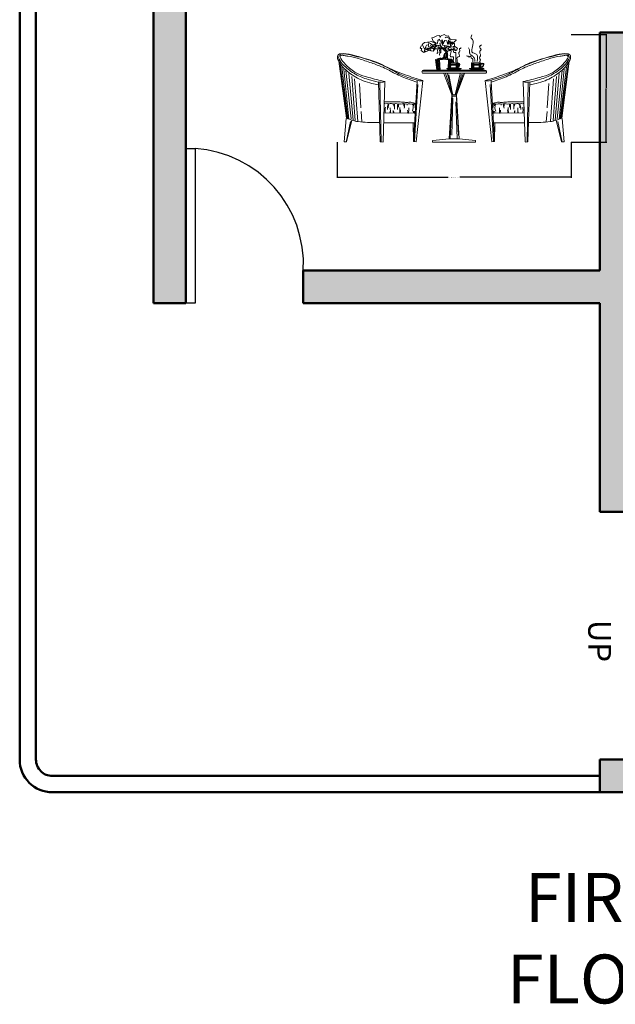
# Model space of a CAD drawing. Units: inches. Extents: x 1771 to 3025, y 319 to 889.
# Tile 13 of 35: x 2219 to 2402, y 319 to 621. Entities that reach past the tile are written whole.
import ezdxf

# ---------------------------------------------------------------- set-up
doc = ezdxf.new("R2010")
doc.units = ezdxf.units.IN
doc.header["$MEASUREMENT"] = 0
for name, color, linetype, lineweight in [('A-ANNO-DIMS', 2, 'Continuous', 18), ('A-AREA-IDEN', 241, 'Continuous', 25), ('A-DOOR', 4, 'Continuous', 25), ('A-FURN', 8, 'Continuous', 18), ('A-WALL', 7, 'Continuous', 50), ('A-WALL-PATT', 254, 'Continuous', 13)]:
    doc.layers.add(name, color=color, linetype=linetype, lineweight=lineweight)
doc.styles.get("Standard").update_dxf_attribs({"font": 'arial.ttf'})
doc.dimstyles.get("Standard").update_dxf_attribs({"dimtxt": 0.18, "dimasz": 0.18, "dimexe": 0.18, "dimexo": 0.0625, "dimgap": 0.09, "dimtad": 0, "dimtih": 1, "dimtoh": 1, "dimdec": 4, "dimzin": 0, "dimdsep": 46, "dimtxsty": 'Standard', "dimcen": 0.09, "dimadec": 0, "dimazin": 0, "dimtfac": 1, "dimtdec": 4, "dimtofl": 0, "dimtmove": 0, "dimatfit": 3, "dimfxl": 1, "dimtolj": 1, "dimtzin": 0, "dimarcsym": 0})

# ---------------------------------------------------------------- blocks, each defined once
blk = doc.blocks.new('A$C7D4176DC')
for p, q in [((850.3, 971.5), (825.9, 951.9)), ((879.3, 973.4), (850.3, 971.5)), ((889.6, 974.3), (879.3, 973.4)), ((886.8, 949.1), (892.4, 968.7)), ((914, 980.9), (889.6, 974.3)), ((892.4, 968.7), (908.4, 962.2)), ((908.4, 962.2), (934.6, 940.6)), ((947.7, 967.8), (914, 980.9)), ((936.5, 1019.3), (919.6, 1018.3)), ((919.6, 1018.3), (933.7, 984.6)), ((933.7, 984.6), (961.8, 966.8)), ((969.3, 1036.1), (936.5, 1019.3)), ((958, 965.9), (946.8, 953.7)), ((961.8, 966.8), (976.7, 961.2)), ((994.5, 1040.8), (969.3, 1036.1)), ((976.7, 961.2), (980.5, 991.2)), ((980.5, 991.2), (994.5, 1005.2)), ((1000.2, 1022.1), (994.5, 1040.8)), ((994.5, 1005.2), (999.2, 992.1)), ((999.2, 992.1), (1006.7, 983.7)), ((999.2, 965.9), (1016.1, 967.8)), ((1003, 952.8), (999.2, 965.9)), ((1008.6, 1036.1), (1000.2, 1022.1)), ((1006.7, 983.7), (1022.6, 987.4)), ((1010.5, 1037.1), (1041.4, 1048.3)), ((1022.6, 987.4), (1015.2, 989.3)), ((1016.1, 967.8), (1017, 970.6)), ((1029.2, 982.8), (1017, 998.7)), ((1017, 998.7), (1017, 981.8)), ((1017, 981.8), (1024.5, 946.2)), ((1017, 970.6), (1037.6, 969.7)), ((1032, 956.5), (1029.2, 982.8)), ((1042.3, 979.9), (1032, 956.5)), ((1037.6, 969.7), (1033, 971.5)), ((1041.4, 1048.3), (1064.8, 1036.1)), ((1047.9, 992.1), (1042.3, 979.9)), ((1066.7, 989.3), (1047.9, 992.1)), ((1051.7, 1018.3), (1059.2, 1023)), ((1059.2, 1023), (1090.1, 1013.6)), ((1064.8, 1036.1), (1077, 1034.2)), ((1075.1, 953.7), (1066.7, 989.3)), ((1077, 1034.2), (1084.5, 1035.2)), ((1081.7, 994), (1079.8, 959.4)), ((1095.7, 976.2), (1081.7, 994)), ((1084.5, 1035.2), (1097.6, 1007.1)), ((1103.2, 982.8), (1084.5, 969.7)), ((1084.5, 969.7), (1084.5, 959.4)), ((1091, 1009.9), (1088.2, 1005.2)), ((1088.2, 1005.2), (1104.1, 1009)), ((1090.1, 1013.6), (1091, 1009.9)), ((1104.1, 1009), (1091, 1005.2)), ((1091, 1005.2), (1100.4, 1003.4)), ((1121, 975.3), (1095.7, 976.2)), ((1100.4, 1003.4), (1103.2, 993.1)), ((1100.4, 971.5), (1103.2, 982.8)), ((1101.3, 940.6), (1100.4, 971.5)), ((1106, 966.8), (1104.1, 968.7)), ((1121, 969.7), (1106, 966.8)), ((1108.2, 1001.8), (1157.5, 996.8)), ((1119.1, 963.1), (1121, 969.7)), ((1127.6, 960.3), (1119.1, 963.1)), ((1132.2, 960.3), (1121, 975.3)), ((1137.9, 978.1), (1132.2, 960.3)), ((1151, 989.3), (1137.9, 978.1)), ((1159.4, 994), (1151, 989.3)), ((1157.5, 996.8), (1159.4, 994)), ((820.3, 941.6), (808.1, 920)), ((808.1, 920), (811.9, 913.5)), ((811.9, 913.5), (821.2, 911.6)), ((821.2, 911.6), (817.5, 893.8)), ((817.5, 893.8), (843.7, 875.1)), ((825.9, 951.9), (853.1, 902.3)), ((843.7, 875.1), (847.5, 880.7)), ((847.5, 897.6), (877.4, 906)), ((847.5, 880.7), (847.5, 897.6)), ((853.1, 902.3), (863.4, 931.3)), ((862.1, 880.4), (853.9, 886.5)), ((860.6, 917.2), (858.7, 916.3)), ((863.4, 917.2), (860.6, 917.2)), ((878.4, 916.3), (861.5, 919.1)), ((886.7, 892.7), (862.1, 880.4)), ((863.4, 931.3), (869, 944.4)), ((876.5, 911.6), (863.4, 917.2)), ((870.3, 898.8), (868.3, 907)), ((869, 944.4), (886.8, 949.1)), ((895, 892.7), (870.3, 898.8)), ((879.3, 906.9), (876.5, 911.6)), ((877.4, 906), (884.9, 905.1)), ((883.1, 912.5), (878.4, 916.3)), ((894.3, 912.5), (879.3, 906.9)), ((910.2, 917.2), (883.1, 912.5)), ((890.6, 924.7), (884, 950)), ((884.9, 905.1), (889.6, 903.2)), ((889.6, 903.2), (895.2, 901.3)), ((900.9, 928.5), (890.6, 924.7)), ((902.7, 916.3), (894.3, 912.5)), ((931.9, 888.6), (895, 892.7)), ((895.2, 901.3), (899, 917.2)), ((922.4, 927.5), (900.9, 928.5)), ((903.7, 927.5), (902.7, 916.3)), ((905.6, 928.5), (903.7, 927.5)), ((904.6, 923.8), (905.6, 928.5)), ((904.6, 920), (904.6, 923.8)), ((919.6, 920), (904.6, 920)), ((909.3, 913.2), (907.3, 892.7)), ((909.3, 940.6), (908.4, 947.2)), ((917.7, 936), (909.3, 940.6)), ((917.5, 890.6), (909.3, 890.6)), ((939.3, 910.7), (910.2, 917.2)), ((931.9, 888.6), (917.5, 890.6)), ((928, 933.1), (917.7, 936)), ((939.3, 913.5), (919.6, 920)), ((932.7, 929.4), (922.4, 927.5)), ((927.4, 947.9), (955.2, 956.5)), ((942.1, 925.7), (928, 933.1)), ((940.1, 909.1), (931.9, 888.6)), ((950.4, 907), (931.9, 888.6)), ((941.1, 929.4), (932.7, 929.4)), ((934.6, 940.6), (938.3, 938.8)), ((985.2, 912.5), (939.3, 910.7)), ((951.5, 911.6), (941.1, 929.4)), ((950.5, 917.2), (942.1, 925.7)), ((946.8, 953.7), (945.8, 946.2)), ((945.8, 946.2), (971.1, 945.3)), ((955.2, 940.6), (946.8, 924.7)), ((946.8, 924.7), (951.5, 918.2)), ((1026.4, 913.5), (950.4, 907.4)), ((952.4, 910.7), (950.5, 917.2)), ((959.9, 938.8), (951.5, 925.7)), ((951.5, 925.7), (954.3, 912.5)), ((951.5, 918.2), (951.5, 911.6)), ((954.3, 909.7), (955.2, 940.6)), ((954.3, 912.5), (954.3, 909.7)), ((955.2, 956.5), (961.8, 934.1)), ((986.1, 943.4), (960.8, 940.6)), ((961.8, 934.1), (984.2, 923.8)), ((967.4, 939.2), (999.2, 945.3)), ((977.6, 875.3), (973.4, 867.6)), ((973.4, 867.6), (973.4, 860.6)), ((976.2, 896.9), (974.8, 892)), ((974.8, 892), (977.6, 877.4)), ((978.3, 903.2), (976.2, 896.9)), ((977.6, 912.2), (978.3, 903.2)), ((977.6, 877.4), (977.6, 875.3)), ((984.2, 923.8), (995.5, 925.7)), ((988.9, 914.4), (985.2, 912.5)), ((989.9, 930.3), (986.1, 943.4)), ((991.7, 916.3), (988.9, 914.4)), ((989.5, 915.7), (998.5, 919.9)), ((995.5, 925.7), (989.9, 930.3)), ((1005.8, 917.2), (991.7, 916.3)), ((998.5, 904.6), (995.7, 898.3)), ((995.7, 898.3), (999.9, 878.8)), ((997.1, 872.5), (996.4, 855.8)), ((999.9, 878.8), (997.1, 872.5)), ((998.5, 919.9), (1000.6, 912.2)), ((1000.6, 912.2), (998.5, 904.6)), ((999.2, 945.3), (1003, 952.8)), ((1002, 948.1), (1001.1, 940.6)), ((1001.1, 940.6), (1006.7, 926.6)), ((1012.3, 931.3), (1002, 948.1)), ((1006.9, 906), (1004.1, 898.3)), ((1004.1, 898.3), (1009, 894.8)), ((1008.3, 872.5), (1004.8, 871.8)), ((1007.7, 920), (1005.8, 917.2)), ((1006.7, 926.6), (1011.4, 921.9)), ((1011.8, 911.5), (1006.9, 906)), ((1006.9, 911.5), (1030.6, 908)), ((1009, 889.2), (1006.9, 877.4)), ((1006.9, 877.4), (1008.3, 872.5)), ((1027.3, 916.3), (1007.7, 920)), ((1009, 894.8), (1009, 889.2)), ((1009.7, 920.6), (1011.8, 911.5)), ((1011.4, 921.9), (1025.5, 914.4)), ((1021.7, 921.9), (1012.3, 931.3)), ((1033, 919.1), (1021.7, 921.9)), ((1024.5, 946.2), (1082.6, 936)), ((1025.5, 914.4), (1048.9, 908.8)), ((1030.6, 908), (1036.9, 901.1)), ((1046.7, 908.7), (1033, 919.1)), ((1036.9, 901.1), (1049.5, 899)), ((1039, 899), (1045.3, 891.3)), ((1049.5, 899), (1039, 899)), ((1047.9, 941.6), (1043.3, 939.7)), ((1043.3, 939.7), (1048.9, 920)), ((1050.9, 864.8), (1044.6, 864.1)), ((1045.3, 891.3), (1052.3, 886.4)), ((1055.4, 914.4), (1047.9, 941.6)), ((1048.9, 920), (1049.8, 910.7)), ((1048.9, 908.8), (1076, 881.7)), ((1049.8, 910.7), (1050.8, 902.3)), ((1050.8, 902.3), (1060.1, 872.3)), ((1058.2, 880.7), (1050.8, 894.8)), ((1055.8, 873.9), (1050.9, 864.8)), ((1052.3, 886.4), (1057.9, 876.7)), ((1067.6, 934.1), (1054.5, 910.7)), ((1054.5, 910.7), (1054.5, 898.5)), ((1054.5, 898.5), (1059.9, 896.9)), ((1056.4, 890.1), (1055.4, 914.4)), ((1056.4, 905.1), (1055.4, 895.7)), ((1055.4, 895.7), (1057.3, 892)), ((1057.9, 876.7), (1055.8, 873.9)), ((1061.1, 918.2), (1056.4, 905.1)), ((1064.4, 865.4), (1056.9, 822.4)), ((1060.1, 872.3), (1058.2, 880.7)), ((1069.5, 859.2), (1059.2, 870.4)), ((1064.8, 923.8), (1061.1, 918.2)), ((1065.7, 884.5), (1061.1, 875.1)), ((1061.1, 875.1), (1061.1, 857.3)), ((1067.6, 929.4), (1064.8, 927.5)), ((1066.7, 926.6), (1064.8, 923.8)), ((1074.2, 859.2), (1065.7, 884.5)), ((1070.4, 864.8), (1065.7, 823.6)), ((1089.2, 931.3), (1066.7, 926.6)), ((1084.5, 932.2), (1067.6, 929.4)), ((1070.4, 862.9), (1067.6, 890.1)), ((1076, 851.7), (1070.4, 864.8)), ((1076, 881.7), (1071.4, 876)), ((1071.4, 876), (1073.2, 863.9)), ((1072.3, 910), (1078.2, 913)), ((1091.3, 904.2), (1072.3, 910)), ((1076.7, 886.6), (1073.8, 883.7)), ((1079.8, 959.4), (1075.1, 953.7)), ((1097.2, 895.4), (1076.7, 886.6)), ((1078.2, 913), (1100.1, 932)), ((1082.6, 936), (1096.7, 928.5)), ((1084.5, 959.4), (1127.6, 960.3)), ((1098.6, 893.9), (1089.9, 904.2)), ((1113.3, 911.5), (1091.3, 904.2)), ((1096.7, 928.5), (1101.3, 922.8)), ((1100.1, 932), (1097.2, 927.6)), ((1097.2, 927.6), (1117.7, 930.5)), ((1113.3, 902.7), (1097.2, 895.4)), ((1113.3, 899.8), (1098.6, 893.9)), ((1101.3, 922.8), (1111.6, 941.6)), ((1111.6, 941.6), (1101.3, 940.6)), ((1122.1, 904.2), (1113.3, 911.5)), ((1127.9, 901.3), (1113.3, 899.8)), ((1117.7, 930.5), (1139.6, 927.6)), ((1138.2, 914.4), (1122.1, 904.2)), ((1138.2, 895.4), (1127.9, 901.3)), ((1129.4, 933.4), (1145.5, 933.4)), ((1144, 908.6), (1138.2, 914.4)), ((1151.3, 895.4), (1138.2, 895.4)), ((1151.3, 891), (1144, 908.6)), ((1145.5, 933.4), (1160.1, 923.2)), ((1166, 901.3), (1151.3, 891)), ((1160.1, 923.2), (1166, 918.8)), ((1166, 918.8), (1170.4, 917.3)), ((1170.4, 917.3), (1166, 901.3)), ((13.4, 788.5), (86.9, 232)), ((968.4, 700.9), (955.2, 806.2)), ((955.2, 806.2), (1126.5, 803.3)), ((959.3, 806.1), (972.5, 701.9)), ((965.6, 806.1), (976.7, 700.5)), ((976.6, 787.5), (968.6, 786.7)), ((968.6, 786.7), (971.7, 756.8)), ((991.6, 820.2), (969.9, 808.3)), ((975.3, 805.4), (983, 701.2)), ((979.7, 757.6), (976.6, 787.5)), ((979.4, 811.3), (977.9, 801.1)), ((991.8, 816.4), (978.6, 806.2)), ((985.8, 805.4), (990.6, 701.9)), ((1016.7, 816), (991.6, 820.2)), ((1003.5, 807.6), (991.8, 816.4)), ((996.2, 804.1), (1001.1, 701.9)), ((996.4, 855.8), (996.4, 850.9)), ((996.4, 850.9), (997.8, 845.3)), ((1009.4, 822.3), (1002, 816.4)), ((1002, 816.4), (1054.7, 813.5)), ((1013.7, 810.6), (1003.5, 807.6)), ((1041.6, 819.3), (1013.7, 810.6)), ((1060.6, 835.8), (1015.2, 815.4)), ((1022.3, 819.5), (1016.7, 816)), ((1024.4, 819.5), (1022.3, 819.5)), ((1026.5, 819.5), (1024.4, 819.5)), ((1029.9, 828.6), (1026.5, 819.5)), ((1032, 829.3), (1029.9, 828.6)), ((1033.4, 828.6), (1032, 829.3)), ((1036.9, 832), (1033.4, 828.6)), ((1037.6, 834.1), (1036.9, 832)), ((1044.5, 828.1), (1037.2, 822.3)), ((1037.2, 822.3), (1041.6, 819.3)), ((1039, 850.9), (1037.6, 836.2)), ((1037.6, 836.2), (1037.6, 834.1)), ((1039.7, 853), (1039, 850.9)), ((1044.6, 864.1), (1039.7, 853)), ((1048.9, 832.5), (1044.5, 828.1)), ((1048.1, 856.4), (1045.3, 850.2)), ((1045.3, 850.2), (1045.3, 839)), ((1045.3, 839), (1048.1, 841.1)), ((1048.1, 841.1), (1048.8, 853.7)), ((1048.8, 853.7), (1048.8, 857.1)), ((1057.7, 829.6), (1048.9, 832.5)), ((1049.8, 817.1), (1076, 851.7)), ((1051.7, 827.4), (1049.8, 817.1)), ((1054.7, 813.5), (1057.7, 829.6)), ((1061.1, 857.3), (1064.8, 853.6)), ((1064.8, 853.6), (1069.5, 859.2)), ((1065.7, 823.6), (1077, 814.3)), ((1066.4, 817.9), (1066.4, 812)), ((1066.4, 812), (1075.2, 806.2)), ((1074.2, 829.2), (1070.4, 862.9)), ((1073.2, 863.9), (1074.2, 859.2)), ((1075.2, 806.2), (1073.8, 812)), ((1073.8, 812), (1114.7, 807.6)), ((1077, 814.3), (1074.2, 829.2)), ((1098.2, 804.7), (1077.7, 804.7)), ((1083.8, 803.4), (1080.4, 718.8)), ((1088.8, 774.3), (1088.8, 724.7)), ((1179, 774.3), (1088.8, 774.3)), ((1090.9, 774.1), (1090.9, 725.1)), ((1093.6, 804.7), (1091.9, 774.3)), ((1093.9, 773.8), (1093.9, 725.1)), ((1114.7, 807.6), (1097.2, 801.8)), ((1098.4, 774.1), (1098.4, 724.9)), ((1104, 802), (1101.5, 774.3)), ((1104.1, 773.8), (1104.1, 763.6)), ((1110.9, 799.9), (1108, 774.3)), ((1117.9, 803.4), (1113.7, 774.3)), ((1125, 803.3), (1120, 774.3)), ((1158.2, 773.8), (1158.2, 725.1)), ((1164.1, 773.8), (1164.1, 724.9)), ((1168.6, 774.3), (1168.6, 725.4)), ((1172.9, 774.1), (1172.9, 767.4)), ((1175.9, 774.1), (1175.9, 767.3)), ((1178, 773.8), (1178, 767.2)), ((1179, 767.3), (1179, 774.3)), ((1309.2, 774.3), (1309.2, 724.7)), ((1399.4, 774.3), (1309.2, 774.3)), ((1311, 774.3), (1311, 725)), ((1313.8, 774.6), (1313.8, 724)), ((1318.3, 774.3), (1318.3, 725.2)), ((1324.3, 774.1), (1324.3, 725.5)), ((1331.2, 774.1), (1331.2, 725)), ((1383.9, 774.1), (1383.9, 725.2)), ((1389.2, 774.1), (1389.2, 724.8)), ((1393.7, 774.1), (1393.7, 724.5)), ((1396.6, 774.1), (1396.6, 724.8)), ((1398.3, 774.1), (1398.3, 724.8)), ((1399.4, 724.7), (1399.4, 774.3)), ((2261.7, 788.5), (2188.2, 232)), ((24.7, 755.7), (94.7, 231.2)), ((41.1, 733.1), (100.8, 229.1)), ((61.7, 710.4), (111.1, 223)), ((82.3, 698.1), (131.7, 227.1)), ((1452.4, 690.9), (826.8, 690.9)), ((1438.5, 700.9), (838.5, 700.9)), ((1107.4, 700.9), (968.4, 700.9)), ((971.7, 756.8), (979.7, 757.6)), ((1206.9, 718.8), (1068.5, 718.8)), ((1205.1, 715), (1070.7, 715)), ((1079.9, 707.4), (1079.6, 701.2)), ((1192.2, 706.1), (1080.1, 706.6)), ((1191.5, 704.8), (1081.7, 704.8)), ((1083.3, 700.5), (1083.3, 704.5)), ((1100.8, 759), (1088.8, 759)), ((1088.8, 724.7), (1179, 724.7)), ((1100.8, 751.4), (1090.1, 751.4)), ((1093.2, 718.3), (1093.2, 724.5)), ((1100.8, 763.6), (1100.8, 747.6)), ((1107.3, 763.6), (1100.8, 763.6)), ((1100.8, 747.6), (1107.3, 747.6)), ((1101.3, 745), (1101.3, 740.5)), ((1107.3, 745), (1101.3, 745)), ((1101.3, 740.5), (1107.3, 740.5)), ((1104.1, 747.6), (1104.1, 745)), ((1104.1, 740.5), (1104.1, 724.7)), ((1107.3, 747.6), (1107.3, 763.6)), ((1179, 759), (1107.3, 759)), ((1179, 751.4), (1107.3, 751.4)), ((1107.3, 740.5), (1107.3, 745)), ((1172.9, 762.7), (1172.9, 734.9)), ((1172.9, 732.2), (1172.9, 725.1)), ((1173.3, 725.1), (1173.3, 718.3)), ((1175.9, 762.6), (1175.9, 734.6)), ((1175.9, 731.8), (1175.9, 724.6)), ((1178.3, 762.6), (1178.3, 734.8)), ((1178.3, 731.3), (1178.3, 725.1)), ((1179, 734.4), (1179, 762.7)), ((1179, 724.7), (1179, 731.4)), ((1189, 704.5), (1189, 700.5)), ((1427.3, 718.8), (1288.9, 718.8)), ((1425.4, 715), (1291, 715)), ((1412.6, 706.1), (1300.5, 706.6)), ((1411.9, 704.8), (1302.1, 704.8)), ((1303.7, 700.5), (1303.7, 704.5)), ((1319.1, 759), (1309.2, 759)), ((1309.2, 724.7), (1399.4, 724.7)), ((1319.1, 751.4), (1310.5, 751.4)), ((1313.5, 718.3), (1313.5, 724.5)), ((1319.1, 764.9), (1319.1, 742.2)), ((1323.5, 764.9), (1319.1, 764.9)), ((1319.1, 742.2), (1323.5, 742.2)), ((1319.8, 739.2), (1319.8, 735.6)), ((1322.7, 739.2), (1319.8, 739.2)), ((1319.8, 735.6), (1322.7, 735.6)), ((1322.7, 735.6), (1322.7, 739.2)), ((1323.5, 742.2), (1323.5, 764.9)), ((1399.4, 759), (1323.5, 759)), ((1399.4, 751.4), (1323.5, 751.4)), ((1393.7, 725.1), (1393.7, 718.3)), ((1409.4, 704.5), (1409.4, 700.5)), ((2192.8, 698.1), (2143.4, 227.1)), ((2213.3, 710.4), (2163.9, 223)), ((2233.9, 733.1), (2174.2, 229.1)), ((2250.4, 755.7), (2180.4, 231.2)), ((111.1, 669.3), (152.3, 214.7)), ((137.9, 640.5), (170.8, 210.6)), ((166.7, 615.8), (197.6, 202.4)), ((398.7, 587.3), (417.4, 0.9)), ((413.7, 579.8), (424.7, 0.9)), ((462.3, 591), (443.8, 0.9)), ((776.4, 594.8), (742.7, 4.4)), ((795.6, 597.2), (767.4, 606)), ((832.5, 602.2), (768.9, 2.8)), ((772.6, 598.5), (776.4, 598.5)), ((825, 598.5), (795.6, 597.2)), ((1438.5, 670.9), (838.5, 670.9)), ((1037.2, 670.1), (1115.4, 459.8)), ((1054.9, 670.7), (1122.1, 460.1)), ((1073, 665.2), (1125.7, 463.7)), ((1085.8, 656.2), (1122.1, 471)), ((1198.4, 667), (1147.5, 461.9)), ((1209.3, 659.8), (1156.6, 467.4)), ((1227.5, 665.2), (1160.2, 467.4)), ((1239.7, 670.1), (1161.5, 459.8)), ((1442.6, 602.2), (1506.2, 2.8)), ((1450.1, 598.5), (1479.4, 597.2)), ((1479.4, 597.2), (1507.7, 606)), ((1502.4, 598.5), (1498.7, 598.5)), ((1498.7, 594.8), (1532.3, 4.4)), ((1812.8, 591), (1831.2, 0.9)), ((1861.4, 579.8), (1850.3, 0.9)), ((1876.4, 587.3), (1857.7, 0.9)), ((2108.4, 615.8), (2077.5, 202.4)), ((2137.2, 640.5), (2104.3, 210.6)), ((2163.9, 669.3), (2122.8, 214.7)), ((214, 572.6), (228.4, 334)), ((783.9, 560.6), (752.8, 5.4)), ((1491.2, 560.6), (1522.3, 5.4)), ((2061, 572.6), (2046.6, 334)), ((1115.4, 459.8), (1088.3, 33.1)), ((1118.5, 442), (1100.3, 33.5)), ((1163.9, 447.4), (1114.8, 447.4)), ((1161.5, 459.8), (1115.4, 459.8)), ((1123.9, 427.4), (1116.6, 68)), ((1154.8, 393), (1167.5, 35.4)), ((1160.2, 436.5), (1180.2, 66.2)), ((1161.5, 459.8), (1188.6, 33.1)), ((230.5, 299.1), (238.7, 196.2)), ((465.7, 375.8), (456.5, 375.8)), ((484.1, 377.3), (471.9, 374.3)), ((499.5, 372.7), (484.1, 377.3)), ((508.7, 374.3), (499.5, 372.7)), ((513.3, 375.8), (508.7, 374.3)), ((525.5, 375.8), (513.3, 375.8)), ((531.7, 374.3), (525.5, 375.8)), ((543.9, 374.3), (531.7, 374.3)), ((547, 371.2), (543.9, 374.3)), ((567, 375.8), (547, 371.2)), ((582.3, 374.3), (567, 375.8)), ((593, 371.2), (590, 374.3)), ((606.8, 372.7), (593, 371.2)), ((611.4, 369.7), (606.8, 372.7)), ((629.8, 372.7), (611.4, 369.7)), ((636, 374.3), (629.8, 372.7)), ((643.6, 375.8), (636, 374.3)), ((648.2, 372.7), (643.6, 375.8)), ((659, 372.7), (648.2, 372.7)), ((677.4, 371.2), (659, 372.7)), ((678.9, 371.2), (678.9, 359)), ((697.3, 374.3), (685.1, 372.7)), ((706.5, 374.3), (697.3, 374.3)), ((715.7, 371.2), (706.5, 374.3)), ((729.5, 372.7), (715.7, 371.2)), ((740.3, 374.3), (729.5, 368.2)), ((729.5, 368.2), (729.5, 372.7)), ((747.9, 374.3), (740.3, 374.3)), ((751, 369.7), (747.9, 374.3)), ((760.2, 374.3), (751, 369.7)), ((1514.9, 374.3), (1524.1, 369.7)), ((1524.1, 369.7), (1527.1, 374.3)), ((1527.1, 374.3), (1534.8, 374.3)), ((1534.8, 374.3), (1545.5, 368.2)), ((1545.5, 372.7), (1559.3, 371.2)), ((1545.5, 368.2), (1545.5, 372.7)), ((1559.3, 371.2), (1568.5, 374.3)), ((1568.5, 374.3), (1577.7, 374.3)), ((1577.7, 374.3), (1590, 372.7)), ((1596.2, 371.2), (1596.2, 359)), ((1597.7, 371.2), (1616.1, 372.7)), ((1616.1, 372.7), (1626.8, 372.7)), ((1626.8, 372.7), (1631.4, 375.8)), ((1631.4, 375.8), (1639.1, 374.3)), ((1639.1, 374.3), (1645.2, 372.7)), ((1645.2, 372.7), (1663.6, 369.7)), ((1663.6, 369.7), (1668.2, 372.7)), ((1668.2, 372.7), (1682, 371.2)), ((1682, 371.2), (1685.1, 374.3)), ((1692.8, 374.3), (1708.1, 375.8)), ((1708.1, 375.8), (1728.1, 371.2)), ((1728.1, 371.2), (1731.1, 374.3)), ((1731.1, 374.3), (1743.4, 374.3)), ((1743.4, 374.3), (1749.5, 375.8)), ((1749.5, 375.8), (1761.8, 375.8)), ((1761.8, 375.8), (1766.4, 374.3)), ((1766.4, 374.3), (1775.6, 372.7)), ((1775.6, 372.7), (1790.9, 377.3)), ((1790.9, 377.3), (1803.2, 374.3)), ((1809.3, 375.8), (1818.5, 375.8)), ((2044.6, 299.1), (2036.3, 196.2)), ((84, 230.1), (64.2, 2.8)), ((126, 200.5), (84, 0.3)), ((140.9, 212.8), (88.9, 2.8)), ((756.8, 280.8), (451.1, 284.6)), ((1518.3, 280.8), (1824, 284.6)), ((2134.2, 212.8), (2186.2, 2.8)), ((2149.1, 200.5), (2191.1, 0.3)), ((2191.1, 230.1), (2210.9, 2.8)), ((447.3, 187.5), (757.7, 187.5)), ((739, 187.5), (742.7, 4.4)), ((1827.8, 187.5), (1517.4, 187.5)), ((1536.1, 187.5), (1532.3, 4.4)), ((64.2, 2.8), (88.9, 2.8)), ((417.4, 0.9), (443.8, 0)), ((742.7, 4.4), (746.5, 38)), ((742.7, 4.4), (768.9, 2.8)), ((927.1, 15), (927.1, 0)), ((1088.3, 33.1), (929, 15)), ((1187.5, 31.7), (1087.6, 31.7)), ((1188.6, 33.1), (1348, 15)), ((1348, 15), (1348, 0)), ((1532.3, 4.4), (1506.2, 2.8)), ((1532.3, 4.4), (1528.6, 38)), ((1857.7, 0.9), (1831.3, 0)), ((2210.9, 2.8), (2186.2, 2.8)), ((1348, 0), (927.1, 0))]:
    blk.add_line(p, q)
for centre, radius, start, end in [((838.2, 685.9), 15, 89.02539, 270.97461), ((1069.4, 716.9), 2.21, 114.75071, 294.8305), ((1059.6, 691.4), 25.9, 31.12717, 65.45392), ((1208.6, 696.5), 19, 99.79621, 154.31096), ((1206.2, 716.7), 1.95, 244.55032, 96.50843), ((1289.8, 716.9), 2.21, 114.75071, 294.8305), ((1280, 691.4), 25.9, 31.12717, 65.45392), ((1429, 696.5), 19, 99.79621, 154.31096), ((1426.6, 716.7), 1.95, 244.55032, 96.50843), ((1440.2, 685.9), 15.1, 263.50595, 96.49405), ((421.9, 675.7), 92.7, 253.90068, 295.36386), ((1853.1, 675.7), 92.7, 244.63614, 286.09932), ((665.2, 310.8), 200.4, 171.53233, 187.34342), ((631.7, 325.3), 145, 160.46362, 183.26427), ((661.3, 321.8), 167.8, 162.1481, 175.52768), ((522.1, 292), 10.6, 155.04372, 216.38582), ((746.2, 323.3), 231.2, 177.65923, 189.89094), ((596.6, 305.3), 53.4, 177.23164, 203.39317), ((-475.8, 101.1), 1042.4, 10.14258, 11.10952), ((592, 359.5), 42.9, 161.29008, 193.50095), ((755.4, 341.1), 200.6, 170.95256, 185.34949), ((841.5, 337.8), 255.8, 172.03905, 184.65389), ((943.9, 345.9), 348.8, 175.42446, 180.75439), ((484.6, 319.5), 124.8, 342.71731, 8.30681), ((204.5, 341.5), 411.6, 351.83053, 356.14259), ((590.6, 356.2), 56.7, 354.25823, 16.89433), ((579.3, 354.7), 74.8, 340.32989, 13.94105), ((645.6, 301.5), 39.5, 333.88539, 14.90767), ((494.8, 326.9), 201, 346.57929, 1.64099), ((619.9, 341.7), 118.4, 339.52102, 14.35705), ((682.4, 301.4), 59.8, 341.0378, 359.49279), ((693.6, 357.6), 48.4, 353.58471, 16.22063), ((616.9, 303.9), 135.6, 349.74606, 359.61704), ((689.2, 351.2), 68.2, 347.09902, 16.48344), ((1585.8, 351.2), 68.2, 163.51656, 192.90098), ((1658.2, 303.9), 135.6, 180.38296, 190.25394), ((1592.7, 301.4), 59.8, 180.50721, 198.9622), ((1581.5, 357.6), 48.4, 163.77937, 186.41529), ((1655.1, 341.7), 118.4, 165.64295, 200.47898), ((1780.3, 326.9), 201, 178.35901, 193.42071), ((1629.4, 301.5), 39.5, 165.09233, 206.11461), ((1695.8, 354.7), 74.8, 166.05895, 199.67011), ((1684.4, 356.2), 56.7, 163.10567, 185.74177), ((2070.6, 341.5), 411.6, 183.85741, 188.16947), ((1790.4, 319.5), 124.8, 171.69319, 197.28269), ((1331.2, 345.9), 348.8, 359.24561, 4.57554), ((1433.6, 337.8), 255.8, 355.34611, 7.96095), ((1519.7, 341.1), 200.6, 354.65051, 9.04744), ((1683.1, 359.5), 42.9, 346.49905, 18.70992), ((2750.9, 101.1), 1042.4, 168.89048, 169.85742), ((1678.5, 305.3), 53.4, 336.60683, 2.76836), ((1528.9, 323.3), 231.2, 350.10906, 2.34077), ((1753, 292), 10.6, 323.61418, 24.95628), ((1613.7, 321.8), 167.8, 4.47232, 17.8519), ((1643.3, 325.3), 145, 356.73573, 19.53638), ((1609.9, 310.8), 200.4, 352.65658, 8.46767)]:
    blk.add_arc(centre, radius, start, end)
for points, knots in [([(1154.2, 782.2), (1154.8, 800.5), (1155.7, 825.5), (1152.5, 852.8), (1161, 880.4), (1126, 866.1), (1137.2, 896.5), (1131.8, 923.4), (1156.8, 968.1), (1113.4, 971.1), (1116.9, 957), (1118.7, 949.8)], [0, 0, 0, 0, 53.324624, 72.369114, 91.413604, 110.471764, 134.594802, 149.830446, 204.42477, 220.941926, 238.716972, 238.716972, 238.716972, 238.716972]), ([(1361.4, 785.9), (1364, 797.1), (1369.1, 819), (1366.1, 867.4), (1305.9, 865.7), (1312.3, 906.5), (1315.7, 942.7), (1336.1, 991.6), (1296, 1015.4), (1304.6, 1034), (1310, 1045.7)], [0, 0, 0, 0, 35.255511, 69.327341, 124.802742, 145.944632, 176.486081, 244.459642, 263.687549, 295.971636, 295.971636, 295.971636, 295.971636]), ([(832.5, 602.2), (773.3, 619.4), (552.4, 683.6), (381.9, 796.6), (-38, 894.8), (125.3, 689.4), (274.3, 633.7), (409.7, 603.5), (466, 591)], [0, 0, 0, 0, 179.241333, 669.878405, 853.517726, 978.360591, 1217.111989, 1387.04363, 1387.04363, 1387.04363, 1387.04363]), ([(1131.4, 779.6), (1130.3, 791.6), (1128.8, 807.5), (1135.2, 839.3), (1091.9, 821.5), (1105.3, 863.2), (1115.5, 900.9), (1079.7, 883.7), (1089.8, 909.5), (1078.6, 906.7), (1072.9, 905.3)], [0, 0, 0, 0, 39.358681, 52.054923, 76.195091, 115.553772, 137.137409, 158.736993, 171.43349, 184.13893, 184.13893, 184.13893, 184.13893]), ([(1166.9, 779.6), (1167.6, 787.2), (1168.9, 801.7), (1159.5, 831.3), (1208.7, 829.6), (1171.7, 871.4), (1202, 885.9), (1182.6, 918), (1207, 909.8), (1204.8, 918.7), (1203.8, 923.1)], [0, 0, 0, 0, 24.123038, 45.706674, 71.213394, 110.655389, 125.899008, 152.561192, 162.725628, 172.882723, 172.882723, 172.882723, 172.882723]), ([(1341.7, 785.9), (1340.2, 798.9), (1337.5, 822.1), (1313, 843.2), (1292.5, 855.8), (1286.2, 880.3), (1292.2, 903.3), (1280.3, 916.5), (1276.7, 920.3)], [0, 0, 0, 0, 37.360481, 67.270583, 93.998428, 104.993238, 141.362472, 156.467713, 156.467713, 156.467713, 156.467713]), ([(1385.6, 784.4), (1390.4, 789.9), (1401.4, 802.3), (1375.2, 822.1), (1401.7, 842.3), (1389.4, 864.6), (1386.5, 887), (1411.5, 904.8), (1373.5, 930.7), (1394.6, 942.4), (1403.7, 947.5)], [0, 0, 0, 0, 18.925439, 42.566292, 64.867201, 90.936936, 109.058775, 128.752565, 161.181972, 185.77482, 185.77482, 185.77482, 185.77482]), ([(1442.6, 602.2), (1501.7, 619.4), (1722.7, 683.6), (1893.2, 796.6), (2313.1, 894.8), (2149.7, 689.4), (2000.7, 633.7), (1865.4, 603.5), (1809.1, 591)], [0, 0, 0, 0, 179.241333, 669.878405, 853.517726, 978.360591, 1217.111989, 1387.04363, 1387.04363, 1387.04363, 1387.04363]), ([(398, 584.9), (364.8, 593.1), (288.2, 612.1), (173, 656.7), (78.3, 727.2), (27.8, 785.3), (-11.1, 856.8), (24.4, 860.7), (34.5, 861.8)], [0, 0, 0, 0, 102.450812, 236.341037, 372.740804, 434.264952, 500.538568, 526.867635, 526.867635, 526.867635, 526.867635]), ([(397.9, 557.5), (377.2, 562.2), (327.1, 573.6), (252, 594.7), (177.4, 633.5), (110.3, 676.9), (52.9, 727.5), (17.7, 778.4), (-3, 818.5), (1.2, 838.8), (2.4, 844.5)], [0, 0, 0, 0, 63.757158, 154.207673, 233.111021, 314.773872, 393.990027, 459.45949, 503.309158, 520.507412, 520.507412, 520.507412, 520.507412]), ([(774.4, 584.9), (749.6, 592.8), (676.5, 616.3), (565.4, 663.8), (449, 732.3), (326.3, 773), (214.5, 813.5), (122.5, 837.9), (67.5, 840.8), (36.8, 851.9), (27.3, 839.8), (24.3, 836)], [0, 0, 0, 0, 78.234212, 230.212389, 361.399227, 482.184421, 615.817971, 721.353317, 759.79292, 789.08251, 802.845503, 802.845503, 802.845503, 802.845503]), ([(778, 604.3), (747.1, 612.4), (671.2, 632.3), (544.7, 691), (406.7, 777.8), (262.4, 816.3), (152.4, 843.8), (83.7, 860.5), (45.9, 861.5), (34.5, 861.8)], [0, 0, 0, 0, 95.639299, 234.867324, 416.660896, 581.537135, 678.863317, 758.06805, 792.133261, 792.133261, 792.133261, 792.133261]), ([(1319.1, 782.9), (1321.9, 795.4), (1325.6, 812.1), (1309.5, 816.4), (1302.3, 822.2), (1305.8, 830.8), (1295.5, 845.6), (1286, 822.9), (1281.2, 839.2), (1270.5, 838.4), (1264.1, 839.6), (1260.1, 840.3)], [0, 0, 0, 0, 30.24085, 40.376736, 46.786017, 54.336911, 66.135106, 80.063877, 89.736225, 97.441532, 109.625491, 109.625491, 109.625491, 109.625491]), ([(1399.4, 767.3), (1402.9, 767.5), (1411.4, 768.1), (1432.6, 770.2), (1424.9, 746.9), (1419.3, 731), (1409, 728.9), (1399.9, 726.6), (1399.4, 728.7), (1399.4, 728.8)], [0, 0, 0, 0, 11.082717, 27.168464, 47.8303, 63.341794, 75.5235, 81.952599, 82.221535, 82.221535, 82.221535, 82.221535]), ([(1497.1, 604.3), (1528, 612.4), (1603.8, 632.3), (1730.4, 691), (1868.3, 777.8), (2012.7, 816.3), (2122.7, 843.8), (2191.4, 860.5), (2229.2, 861.5), (2240.6, 861.8)], [0, 0, 0, 0, 95.639299, 234.867324, 416.660896, 581.537135, 678.863317, 758.06805, 792.133261, 792.133261, 792.133261, 792.133261]), ([(1500.6, 584.9), (1525.5, 592.8), (1598.5, 616.3), (1709.7, 663.8), (1826.1, 732.3), (1948.7, 773), (2060.6, 813.5), (2152.5, 837.9), (2207.6, 840.8), (2238.3, 851.9), (2247.7, 839.8), (2250.7, 836)], [0, 0, 0, 0, 78.234212, 230.212389, 361.399227, 482.184421, 615.817971, 721.353317, 759.79292, 789.08251, 802.845503, 802.845503, 802.845503, 802.845503]), ([(1877.1, 584.9), (1910.3, 593.1), (1986.9, 612.1), (2102.1, 656.7), (2196.8, 727.2), (2247.3, 785.3), (2286.2, 856.8), (2250.7, 860.7), (2240.6, 861.8)], [0, 0, 0, 0, 102.450812, 236.341037, 372.740804, 434.264952, 500.538568, 526.867635, 526.867635, 526.867635, 526.867635]), ([(1877.1, 557.5), (1897.9, 562.2), (1947.9, 573.6), (2023.1, 594.7), (2097.7, 633.5), (2164.7, 676.9), (2222.2, 727.5), (2257.3, 778.4), (2278.1, 818.5), (2273.8, 838.8), (2272.7, 844.5)], [0, 0, 0, 0, 63.757158, 154.207673, 233.111021, 314.773872, 393.990027, 459.45949, 503.309158, 520.507412, 520.507412, 520.507412, 520.507412]), ([(1169.5, 767.6), (1169.1, 766.9), (1168.6, 765.8), (1168.5, 764.1), (1168.9, 763.4), (1169.1, 763)], [0, 0, 0, 0, 2.454471, 3.694729, 4.863756, 4.863756, 4.863756, 4.863756]), ([(1169.1, 763), (1172.8, 762.7), (1177.7, 762.3), (1183.6, 763.4), (1189.9, 762.9), (1187.4, 754.3), (1187.2, 747.1), (1184.4, 741.1), (1183.6, 734.2), (1179.1, 734.3), (1176.3, 734.5), (1173.7, 734.9), (1171.6, 734.9), (1169.1, 736.3), (1168.8, 734.4), (1168.7, 733.5), (1168.7, 732.9), (1169, 732.2), (1169.6, 732.2), (1169.9, 732.3)], [0, 0, 0, 0, 11.017731, 14.368752, 18.607743, 26.502791, 33.640107, 41.65747, 47.330925, 50.070533, 53.653147, 56.161165, 57.765785, 60.50412, 61.601302, 62.440841, 63.254964, 63.604793, 64.589255, 64.589255, 64.589255, 64.589255]), ([(1169.5, 767.6), (1173.2, 767.4), (1179.9, 766.9), (1197.8, 769.9), (1190.9, 747.3), (1187.7, 728.5), (1175.3, 732.4), (1169.7, 732.3), (1169.1, 732.2)], [0, 0, 0, 0, 11.640419, 20.980802, 45.0396, 57.043585, 71.929427, 73.92866, 73.92866, 73.92866, 73.92866]), ([(1180.5, 766.4), (1182.7, 766.7), (1186, 767.2), (1193.4, 764.4), (1189.7, 753.8), (1188.7, 747.3), (1188.2, 744.3)], [0, 0, 0, 0, 6.446326, 10.075492, 21.292554, 31.027811, 31.027811, 31.027811, 31.027811]), ([(1399.4, 760.8), (1402.3, 761.2), (1409.4, 762.1), (1423.2, 766.3), (1423.3, 753.9), (1420.3, 746.4), (1417.8, 735.7), (1409.3, 733.5), (1403.3, 729.7), (1400.4, 731.6), (1399.4, 732.3)], [0, 0, 0, 0, 9.652474, 22.996839, 29.518582, 40.146055, 49.702279, 58.739504, 65.130432, 68.539734, 68.539734, 68.539734, 68.539734]), ([(763.3, 374.3), (771.1, 374), (721.2, 391.5), (701, 387.4), (647.2, 387.1), (600.7, 394.2), (547.4, 391.8), (499.5, 394.7), (467.3, 394.3), (453.5, 394.2)], [0, 0, 0, 0, 23.359127, 69.600901, 112.546095, 167.952511, 215.499051, 270.735631, 312.147322, 312.147322, 312.147322, 312.147322]), ([(1511.8, 374.3), (1504, 374), (1553.9, 391.5), (1574.1, 387.4), (1627.8, 387.1), (1674.4, 394.2), (1727.7, 391.8), (1775.6, 394.7), (1807.8, 394.3), (1821.6, 394.2)], [0, 0, 0, 0, 23.359127, 69.600901, 112.546095, 167.952511, 215.499051, 270.735631, 312.147322, 312.147322, 312.147322, 312.147322]), ([(86.9, 232), (124.5, 219.1), (220.3, 186.2), (332, 194.5), (402.2, 190.3), (411.4, 189.7)], [0, 0, 0, 0, 118.259021, 301.591906, 329.266035, 329.266035, 329.266035, 329.266035]), ([(2188.2, 232), (2150.6, 219.1), (2054.8, 186.2), (1943.1, 194.5), (1872.9, 190.3), (1863.7, 189.7)], [0, 0, 0, 0, 118.259021, 301.591906, 329.266035, 329.266035, 329.266035, 329.266035])]:
    blk.add_open_spline(points, degree=3, knots=knots)
blk = doc.blocks.new('DOOR-36A')
blk.add_lwpolyline([(0, 47.37), (2.84, 47.37), (2.84, 0), (0, 0)], close=True)
blk.add_arc((0.47, 11.87), 35.58, 356.991, 86.1899)
blk = doc.blocks.new('*D44')
at = {"layer": 'A-ANNO-DIMS', "color": 0, "lineweight": -2, "transparency": 16777216}
for p, q in [((2316.52, 582.92), (2316.52, 572.04)), ((2388.29, 582.92), (2388.29, 572.04)), ((2316.7, 572.22), (2350.62, 572.22)), ((2388.11, 572.22), (2354.19, 572.22))]:
    blk.add_line(p, q, dxfattribs=at)
at = {"layer": 'A-ANNO-DIMS', "color": 0, "transparency": 16777216}
for points in [[(2316.7, 572.25), (2316.7, 572.19), (2316.52, 572.22)], [(2388.11, 572.25), (2388.11, 572.19), (2388.29, 572.22)]]:
    blk.add_solid(points, dxfattribs=at)
at = {"layer": 'Defpoints', "color": 0, "transparency": 16777216}
for p in [(2316.52, 582.99), (2388.29, 582.99), (2388.29, 572.22)]:
    blk.add_point(p, dxfattribs=at)
at = {"layer": 'A-ANNO-DIMS', "color": 0, "transparency": 16777216, "insert": (2352.4, 572.22), "char_height": 0.18, "attachment_point": 5}
blk.add_mtext('\\A1;COFFEE TABLE SET 72 TYP.', dxfattribs=at)
blk = doc.blocks.new('*D45')
at = {"layer": 'A-ANNO-DIMS', "color": 0, "lineweight": -2, "transparency": 16777216}
for p, q in [((2388.35, 615.93), (2399.24, 615.93)), ((2399.06, 615.75), (2399.06, 599.64)), ((2399.06, 583.17), (2399.06, 599.28)), ((2388.35, 582.99), (2399.24, 582.99))]:
    blk.add_line(p, q, dxfattribs=at)
at = {"layer": 'A-ANNO-DIMS', "color": 0, "transparency": 16777216}
for points in [[(2399.03, 615.75), (2399.09, 615.75), (2399.06, 615.93)], [(2399.03, 583.17), (2399.09, 583.17), (2399.06, 582.99)]]:
    blk.add_solid(points, dxfattribs=at)
at = {"layer": 'Defpoints', "color": 0, "transparency": 16777216}
for p in [(2388.29, 615.93), (2399.06, 615.93), (2388.29, 582.99)]:
    blk.add_point(p, dxfattribs=at)
at = {"layer": 'A-ANNO-DIMS', "color": 0, "transparency": 16777216, "insert": (2399.06, 599.46), "char_height": 0.18, "attachment_point": 5}
blk.add_mtext('\\A1;33 TYP.', dxfattribs=at)

msp = doc.modelspace()

# ---------------------------------------------------------------- hatches: boundary and pattern name
at = {"layer": 'A-WALL-PATT'}
h = msp.add_hatch(color=256, dxfattribs=at)
h.dxf.hatch_style = 1
h.paths.add_polyline_path([(2407.16, 878.63), (2429.21, 878.63), (2429.21, 888.63), (2379.16, 888.63), (2379.16, 878.63), (2402.16, 878.63), (2402.16, 830.63), (2407.16, 830.63)])
h.paths.add_polyline_path([(2520.11, 888.63), (2477.21, 888.63), (2477.21, 878.63), (2498.16, 878.63), (2498.16, 794.63), (2402.16, 794.63), (2402.16, 758.63), (2402.16, 664.63), (2407.16, 664.63), (2407.16, 712), (2407.16, 789.63), (2515.16, 789.63), (2515.16, 794.63), (2503.16, 794.63), (2503.16, 878.63), (2520.11, 878.63)])
h.paths.add_polyline_path([(2561.16, 888.63), (2538.11, 888.63), (2538.11, 878.63), (2551.16, 878.63), (2551.16, 789.63), (2551.16, 768.61), (2561.16, 768.61)])
h.paths.add_polyline_path([(2561.16, 720.61), (2551.16, 720.61), (2551.16, 669.63), (2443.16, 669.63), (2443.16, 664.63), (2462.16, 664.63), (2462.16, 652.63), (2467.16, 652.63), (2467.16, 664.63), (2551.16, 664.63), (2551.16, 649.17), (2561.16, 649.17)])
h.paths.add_polyline_path([(2561.16, 631.17), (2551.16, 631.17), (2551.16, 616.63), (2462.16, 616.63), (2443.16, 616.63), (2443.16, 611.63), (2551.16, 611.63), (2551.16, 581.11), (2561.16, 581.11)])
h.paths.add_polyline_path([(2561.16, 533.11), (2551.16, 533.11), (2551.16, 479.63), (2407.16, 479.63), (2407.16, 616.63), (2397.16, 616.63), (2397.16, 543.63), (2306.16, 543.63), (2306.16, 533.63), (2397.16, 533.63), (2397.16, 469.63), (2551.16, 469.63), (2551.16, 452.76), (2561.16, 452.76)])
h.paths.add_polyline_path([(2561.16, 404.76), (2551.16, 404.76), (2551.16, 393.63), (2397.16, 393.63), (2397.16, 383.63), (2561.16, 383.63)])
h.paths.add_polyline_path([(2270.16, 642.58), (2260.16, 642.58), (2260.16, 533.63), (2270.16, 533.63)])
h.paths.add_polyline_path([(2270.16, 753.63), (2366.16, 753.63), (2366.16, 758.63), (2270.16, 758.63), (2270.16, 842.59, -0.008336), (2268.86, 842.63), (2260.16, 842.63), (2260.16, 690.58), (2270.16, 690.58)])
h.paths.add_polyline_path([(2331.16, 888.63), (2260.16, 888.63), (2260.16, 878.63), (2331.16, 878.63)])

# ---------------------------------------------------------------- linework, layer by layer
at = {"layer": 'A-WALL'}
for p, q in [((2219.16, 888.63), (2219.16, 533.63)), ((2224.16, 878.63), (2224.16, 533.63)), ((2260.16, 842.63), (2260.16, 533.63)), ((2270.16, 753.63), (2270.16, 533.63)), ((2407.16, 616.63), (2397.16, 616.63)), ((2397.16, 616.63), (2397.16, 543.63)), ((2397.16, 543.63), (2306.16, 543.63)), ((2306.16, 543.63), (2306.16, 533.63)), ((2270.16, 533.63), (2260.16, 533.63)), ((2397.16, 533.63), (2306.16, 533.63)), ((2397.16, 533.63), (2397.16, 469.63)), ((2397.16, 469.63), (2551.16, 469.63)), ((2397.16, 393.63), (2551.16, 393.63)), ((2397.16, 393.63), (2397.16, 383.63)), ((2397.16, 383.63), (2561.16, 383.63))]:
    msp.add_line(p, q, dxfattribs=at)
for points in [[(2219.16, 533.63), (2219.16, 393.63, 0.414214), (2229.16, 383.63), (2397.16, 383.63)], [(2224.16, 533.63), (2224.16, 393.63, 0.414214), (2229.16, 388.63), (2397.16, 388.63)]]:
    msp.add_lwpolyline(points, format="xyb", dxfattribs=at)

# ---------------------------------------------------------------- block references
at = {"layer": 'A-DOOR'}
msp.add_blockref('DOOR-36A', (2270.16, 533.63), dxfattribs=at)
at = {"layer": 'A-FURN', "xscale": 0.0314240770509951, "yscale": 0.0314240770509951, "zscale": 0.0314240770509951}
msp.add_blockref('A$C7D4176DC', (2316.66, 582.99), dxfattribs=at)

# ---------------------------------------------------------------- texts
at = {"layer": 'A-AREA-IDEN', "insert": (2400.56, 472.75), "char_height": 7, "attachment_point": 1, "rotation": 270}
msp.add_mtext_dynamic_manual_height_columns('\\pxqc;UP', width=85.4611, gutter_width=1, heights=[0], dxfattribs=at)
at = {"layer": 'A-AREA-IDEN', "insert": (2358.75, 358.88), "char_height": 15, "attachment_point": 1}
msp.add_mtext_dynamic_manual_height_columns('\\pxqc;FIRST FLOOR ', width=85.4611, gutter_width=1, heights=[0], dxfattribs=at)

# ---------------------------------------------------------------- dimensions: what is measured, and where the dimension line sits
at = {"layer": 'A-ANNO-DIMS'}
dim = msp.add_linear_dim(base=(2399.06, 615.93), p1=(2388.29, 582.99), p2=(2388.29, 615.93), angle=90, text='<> TYP.', dimstyle='Standard', override={"dimdec": 0, "dimrnd": 0, "dimzin": 0, "dimlunit": 2}, dxfattribs=at)
dim.commit()
dim.dimension.update_dxf_attribs({"geometry": '*D45', "text_midpoint": (2399.06, 599.46)})
dim = msp.add_linear_dim(base=(2388.29, 572.22), p1=(2316.52, 582.99), p2=(2388.29, 582.99), text='COFFEE TABLE SET <> TYP.', dimstyle='Standard', override={"dimdec": 0, "dimrnd": 0, "dimzin": 0, "dimlunit": 2}, dxfattribs=at)
dim.commit()
dim.dimension.update_dxf_attribs({"geometry": '*D44', "text_midpoint": (2352.4, 572.22)})

doc.saveas('drawing.dxf')
